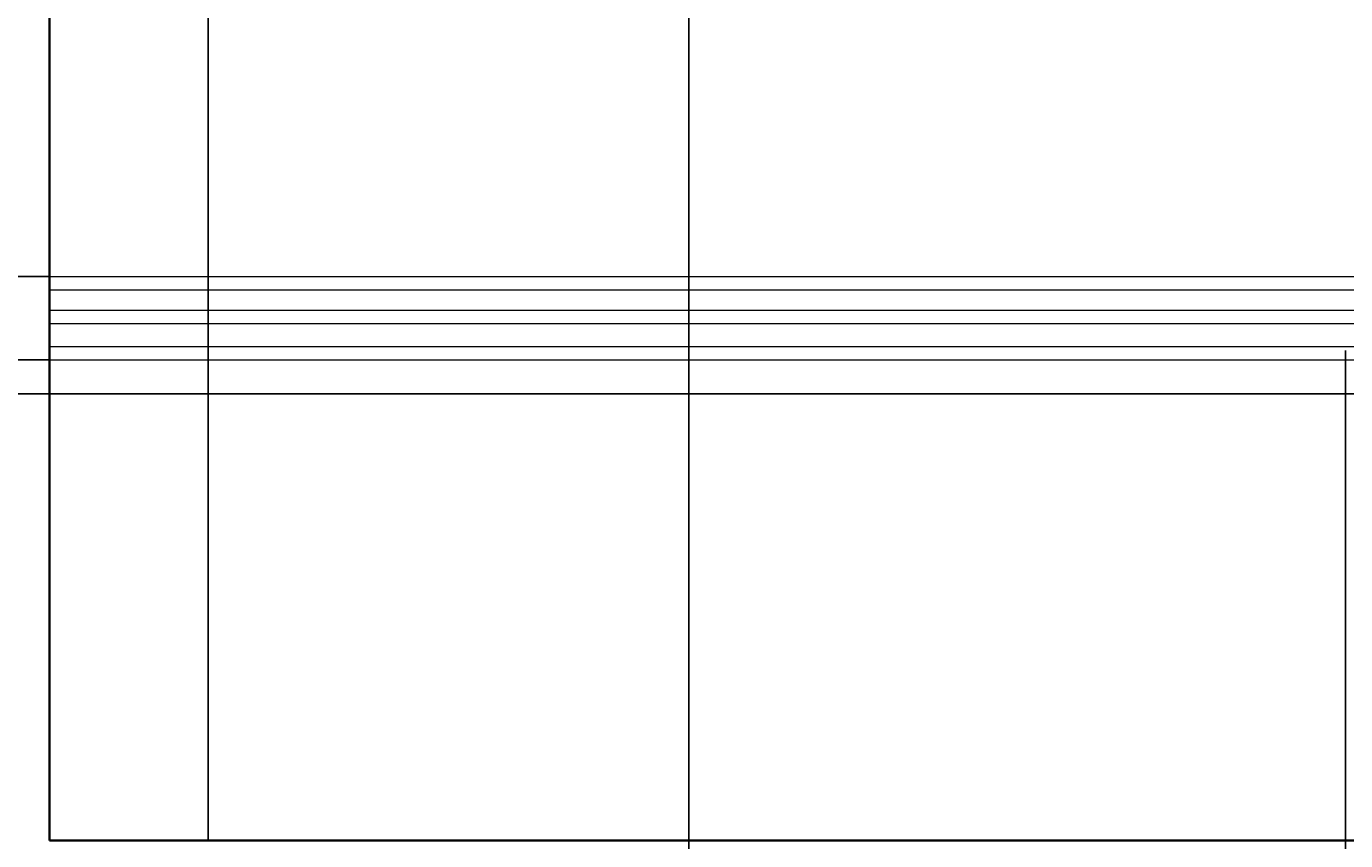
# Model space of a CAD drawing. Units: inches. Extents: x -13 to 809, y 112 to 656.
# Tile 14 of 55: x 111 to 210, y 325 to 385. Entities that reach past the tile are written whole.
import ezdxf

# ---------------------------------------------------------------- set-up
doc = ezdxf.new("R2010")
doc.units = ezdxf.units.IN
doc.header["$MEASUREMENT"] = 0
for name, color, linetype, lineweight in [('A-ANNO-DIMS', 2, 'Continuous', 18), ('A-DOOR', 4, 'Continuous', 25), ('A-ELEV', 7, 'Continuous', 35), ('A-ELEV-PATT', 8, 'Continuous', 13)]:
    doc.layers.add(name, color=color, linetype=linetype, lineweight=lineweight)
doc.styles.get("Standard").update_dxf_attribs({"font": 'arial.ttf'})
doc.dimstyles.get("Standard").update_dxf_attribs({"dimtxt": 0.625, "dimasz": 0.18, "dimexe": 0.18, "dimexo": 0.0625, "dimgap": 0.09, "dimtad": 0, "dimtih": 1, "dimtoh": 1, "dimdec": 4, "dimzin": 0, "dimdsep": 46, "dimlunit": 4, "dimtxsty": 'Standard', "dimcen": 0.09, "dimadec": 0, "dimazin": 0, "dimtfac": 1, "dimtdec": 4, "dimtofl": 0, "dimtmove": 0, "dimatfit": 3, "dimfxl": 1, "dimtolj": 1, "dimtzin": 0, "dimarcsym": 0})

# ---------------------------------------------------------------- blocks, each defined once
blk = doc.blocks.new('*D39')
at = {"layer": 'A-ANNO-DIMS', "color": 0, "lineweight": -2, "transparency": 16777216}
for p, q in [((341.345, 524.281), (-12.099, 524.281)), ((-11.919, 524.101), (-11.919, 406.775)), ((-11.919, 288.631), (-11.919, 405.957)), ((341.345, 288.451), (-12.099, 288.451))]:
    blk.add_line(p, q, dxfattribs=at)
at = {"layer": 'A-ANNO-DIMS', "color": 0, "transparency": 16777216}
for points in [[(-11.949, 524.101), (-11.889, 524.101), (-11.919, 524.281)], [(-11.949, 288.631), (-11.889, 288.631), (-11.919, 288.451)]]:
    blk.add_solid(points, dxfattribs=at)
at = {"layer": 'Defpoints', "color": 0, "transparency": 16777216}
for p in [(-11.919, 524.281), (341.407, 524.281), (341.407, 288.451)]:
    blk.add_point(p, dxfattribs=at)
at = {"layer": 'A-ANNO-DIMS', "color": 0, "transparency": 16777216, "insert": (-11.919, 406.366), "char_height": 0.625, "attachment_point": 5}
blk.add_mtext('\\A1;235.83', dxfattribs=at)
blk = doc.blocks.new('*D41')
at = {"layer": 'A-ANNO-DIMS', "color": 0, "lineweight": -2, "transparency": 16777216}
for p, q in [((471.037, 357.98), (-12.099, 357.98)), ((-11.919, 357.8), (-11.919, 335.983)), ((-11.919, 313.347), (-11.919, 335.164)), ((471.037, 313.167), (-12.099, 313.167))]:
    blk.add_line(p, q, dxfattribs=at)
at = {"layer": 'A-ANNO-DIMS', "color": 0, "transparency": 16777216}
for points in [[(-11.949, 357.8), (-11.889, 357.8), (-11.919, 357.98)], [(-11.949, 313.347), (-11.889, 313.347), (-11.919, 313.167)]]:
    blk.add_solid(points, dxfattribs=at)
at = {"layer": 'Defpoints', "color": 0, "transparency": 16777216}
for p in [(-11.919, 357.98), (471.1, 357.98), (471.1, 313.167)]:
    blk.add_point(p, dxfattribs=at)
at = {"layer": 'A-ANNO-DIMS', "color": 0, "transparency": 16777216, "insert": (-11.919, 335.574), "char_height": 0.625, "attachment_point": 5}
blk.add_mtext('\\A1;44.81', dxfattribs=at)
blk = doc.blocks.new('*D42')
at = {"layer": 'A-ANNO-DIMS', "color": 0, "lineweight": -2, "transparency": 16777216}
for p, q in [((471.037, 414.859), (-12.099, 414.859)), ((-11.919, 414.679), (-11.919, 386.829)), ((-11.919, 358.16), (-11.919, 386.011)), ((471.037, 357.98), (-12.099, 357.98))]:
    blk.add_line(p, q, dxfattribs=at)
at = {"layer": 'A-ANNO-DIMS', "color": 0, "transparency": 16777216}
for points in [[(-11.949, 414.679), (-11.889, 414.679), (-11.919, 414.859)], [(-11.949, 358.16), (-11.889, 358.16), (-11.919, 357.98)]]:
    blk.add_solid(points, dxfattribs=at)
at = {"layer": 'Defpoints', "color": 0, "transparency": 16777216}
for p in [(-11.919, 414.859), (471.1, 414.859), (471.1, 357.98)]:
    blk.add_point(p, dxfattribs=at)
at = {"layer": 'A-ANNO-DIMS', "color": 0, "transparency": 16777216, "insert": (-11.919, 386.42), "char_height": 0.625, "attachment_point": 5}
blk.add_mtext('\\A1;56.88', dxfattribs=at)
blk = doc.blocks.new('*D46')
at = {"layer": 'A-ANNO-DIMS', "color": 0, "lineweight": -2, "transparency": 16777216}
for p, q in [((160.981, 408.794), (807.769, 408.794)), ((807.589, 408.614), (807.589, 367.066)), ((807.589, 324.7), (807.589, 366.248)), ((160.981, 324.52), (807.769, 324.52))]:
    blk.add_line(p, q, dxfattribs=at)
at = {"layer": 'A-ANNO-DIMS', "color": 0, "transparency": 16777216}
for points in [[(807.559, 408.614), (807.619, 408.614), (807.589, 408.794)], [(807.559, 324.7), (807.619, 324.7), (807.589, 324.52)]]:
    blk.add_solid(points, dxfattribs=at)
at = {"layer": 'Defpoints', "color": 0, "transparency": 16777216}
for p in [(160.918, 408.794), (807.589, 408.794), (160.918, 324.52)]:
    blk.add_point(p, dxfattribs=at)
at = {"layer": 'A-ANNO-DIMS', "color": 0, "transparency": 16777216, "insert": (807.589, 366.657), "char_height": 0.625, "attachment_point": 5}
blk.add_mtext('\\A1;84.27', dxfattribs=at)
blk = doc.blocks.new('*D111')
at = {"layer": 'A-ANNO-DIMS', "color": 0, "lineweight": -2, "transparency": 16777216}
for p, q in [((210.079, 361.229), (210.079, 112.34)), ((160.918, 324.457), (160.918, 112.34)), ((161.098, 112.52), (184.342, 112.52)), ((209.899, 112.52), (186.656, 112.52))]:
    blk.add_line(p, q, dxfattribs=at)
at = {"layer": 'A-ANNO-DIMS', "color": 0, "transparency": 16777216}
for points in [[(161.098, 112.55), (161.098, 112.49), (160.918, 112.52)], [(209.899, 112.55), (209.899, 112.49), (210.079, 112.52)]]:
    blk.add_solid(points, dxfattribs=at)
at = {"layer": 'Defpoints', "color": 0, "transparency": 16777216}
for p in [(210.079, 361.292), (160.918, 324.52), (210.079, 112.52)]:
    blk.add_point(p, dxfattribs=at)
at = {"layer": 'A-ANNO-DIMS', "color": 0, "transparency": 16777216, "insert": (185.499, 112.52), "char_height": 0.625, "attachment_point": 5}
blk.add_mtext('\\A1;49.16', dxfattribs=at)
blk = doc.blocks.new('*D112')
at = {"layer": 'A-ANNO-DIMS', "color": 0, "lineweight": -2, "transparency": 16777216}
for p, q in [((210.079, 361.229), (210.079, 112.34)), ((275.715, 361.229), (275.715, 112.34)), ((210.259, 112.52), (241.752, 112.52)), ((275.535, 112.52), (244.042, 112.52))]:
    blk.add_line(p, q, dxfattribs=at)
at = {"layer": 'A-ANNO-DIMS', "color": 0, "transparency": 16777216}
for points in [[(210.259, 112.55), (210.259, 112.49), (210.079, 112.52)], [(275.535, 112.55), (275.535, 112.49), (275.715, 112.52)]]:
    blk.add_solid(points, dxfattribs=at)
at = {"layer": 'Defpoints', "color": 0, "transparency": 16777216}
for p in [(210.079, 361.292), (275.715, 361.292), (275.715, 112.52)]:
    blk.add_point(p, dxfattribs=at)
at = {"layer": 'A-ANNO-DIMS', "color": 0, "transparency": 16777216, "insert": (242.897, 112.52), "char_height": 0.625, "attachment_point": 5}
blk.add_mtext('\\A1;65.64', dxfattribs=at)
blk = doc.blocks.new('*D114')
at = {"layer": 'A-ANNO-DIMS', "color": 0, "lineweight": -2, "transparency": 16777216}
for p, q in [((112.984, 366.753), (-12.099, 366.753)), ((-11.919, 366.573), (-11.919, 364.046)), ((-11.919, 360.7), (-11.919, 363.227)), ((112.984, 360.52), (-12.099, 360.52))]:
    blk.add_line(p, q, dxfattribs=at)
at = {"layer": 'A-ANNO-DIMS', "color": 0, "transparency": 16777216}
for points in [[(-11.949, 366.573), (-11.889, 366.573), (-11.919, 366.753)], [(-11.949, 360.7), (-11.889, 360.7), (-11.919, 360.52)]]:
    blk.add_solid(points, dxfattribs=at)
at = {"layer": 'Defpoints', "color": 0, "transparency": 16777216}
for p in [(113.047, 366.753), (-11.919, 360.52), (113.047, 360.52)]:
    blk.add_point(p, dxfattribs=at)
at = {"layer": 'A-ANNO-DIMS', "color": 0, "transparency": 16777216, "insert": (-11.919, 363.636), "char_height": 0.625, "attachment_point": 5}
blk.add_mtext('\\A1;6.233', dxfattribs=at)

msp = doc.modelspace()

# ---------------------------------------------------------------- linework, layer by layer
at = {"layer": 'A-DOOR'}
for p, q in [((124.9184, 348.7114), (124.9184, 408.7939)), ((160.9184, 408.7939), (160.9184, 348.7114)), ((124.9184, 348.7114), (124.9184, 324.5199)), ((160.9184, 348.7114), (160.9184, 324.5199))]:
    msp.add_line(p, q, dxfattribs=at)
at = {"layer": 'A-ELEV'}
for q in [(113.0469, 444.5199), (319.5074, 324.5199)]:
    msp.add_line((113.0469, 324.5199), q, dxfattribs=at)
at = {"layer": 'A-ELEV-PATT'}
for p, q in [((113.0469, 366.753), (319.5074, 366.753)), ((113.0469, 365.753), (319.5074, 365.753)), ((113.0469, 364.2343), (319.5074, 364.2343)), ((113.0469, 363.2343), (319.5074, 363.2343)), ((113.0469, 361.5199), (319.5074, 361.5199)), ((113.0469, 360.5199), (319.5074, 360.5199))]:
    msp.add_line(p, q, dxfattribs=at)

# ---------------------------------------------------------------- dimensions: what is measured, and where the dimension line sits
at = {"layer": 'A-ANNO-DIMS'}
for base, p1, p2, override, picture, middle in [((-11.9191, 524.281), (341.4072, 288.4508), (341.4072, 524.281), {"dimdec": 2, "dimlfac": 1, "dimrnd": 0, "dimzin": 0, "dimdsep": 46, "dimlunit": 2}, '*D39', (-11.9191, 406.3659)), ((-11.9191, 414.8594), (471.0998, 357.9804), (471.0998, 414.8594), {"dimdec": 2, "dimlfac": 1, "dimrnd": 0, "dimzin": 0, "dimdsep": 46, "dimlunit": 2}, '*D42', (-11.9191, 386.4199)), ((807.5888, 408.7939), (160.9184, 324.5199), (160.9184, 408.7939), {"dimdec": 2, "dimlfac": 1, "dimrnd": 0, "dimzin": 0, "dimdsep": 46, "dimlunit": 2}, '*D46', (807.5888, 366.6569)), ((-11.9191, 360.5199), (113.0469, 366.753), (113.0469, 360.5199), {"dimdec": 3, "dimlfac": 1, "dimrnd": 0, "dimzin": 0, "dimdsep": 46, "dimlunit": 2}, '*D114', (-11.9191, 363.6364)), ((-11.9191, 357.9804), (471.0998, 313.1667), (471.0998, 357.9804), {"dimdec": 2, "dimlfac": 1, "dimrnd": 0, "dimzin": 0, "dimdsep": 46, "dimlunit": 2}, '*D41', (-11.9191, 335.5735))]:
    dim = msp.add_linear_dim(base=base, p1=p1, p2=p2, angle=90, dimstyle='Standard', override=override, dxfattribs=at)
    dim.commit()
    dim.dimension.update_dxf_attribs({"geometry": picture, "text_midpoint": middle})
for base, p1, p2, picture, middle in [((210.0791, 112.5199), (160.9184, 324.5199), (210.0791, 361.2915), '*D111', (185.4988, 112.5199)), ((275.7145, 112.5199), (210.0791, 361.2915), (275.7145, 361.2915), '*D112', (242.8968, 112.5199))]:
    dim = msp.add_linear_dim(base=base, p1=p1, p2=p2, dimstyle='Standard', override={"dimdec": 2, "dimlfac": 1, "dimrnd": 0, "dimzin": 0, "dimdsep": 46, "dimlunit": 2}, dxfattribs=at)
    dim.commit()
    dim.dimension.update_dxf_attribs({"geometry": picture, "text_midpoint": middle})

doc.saveas('drawing.dxf')
